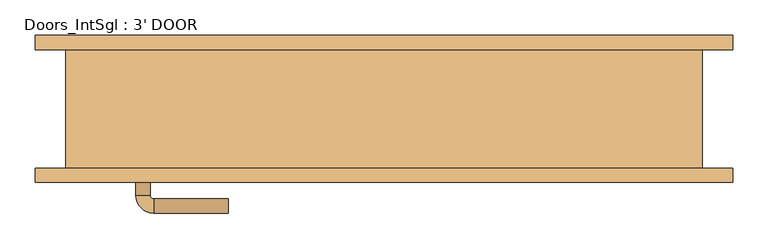
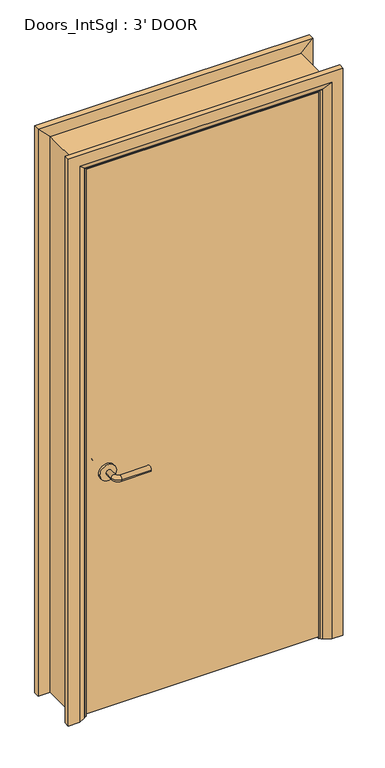
"""IFC4 building model written with IfcOpenShell, lengths in millimetres: door geometry, Doors_IntSgl : 3' DOOR."""

from ifc_helpers import new_model, si_unit, point, frame, frame_2d, origin, place, context, project, spatial, polyline, circle_curve, ellipse_curve, trimmed, segment, composite_curve, outline, extrude, faceted_brep, source, transform, mapped, element, save
from ifc_brep_helpers import plane_surface, cylinder_surface, revolved_surface, advanced_brep


def doors_intsgl_3_door_2f660dd7(model_context):
    return source(origin(), model_context, "Body", "SolidModel", [
        advanced_brep(
        [(-350.2, -37.82, 900.0), (-330.2, -37.82, 900.0), (-350.2, -7.82, 900.0), (-330.2, -7.82, 900.0), (-325.2, -2.82, 900.0), (-325.2, 17.18, 900.0), (-220.2, 17.18, 900.0), (-220.2, -2.82, 900.0)],
        [
            (0, 1, circle_curve(frame((-340.2, -37.82, 900.0), z_axis=(0.0, -1.0, 0.0), x_axis=(1.0, 0.0, 0.0)), 10.0)),
            (1, 0, circle_curve(frame((-340.2, -37.82, 900.0), z_axis=(0.0, -1.0, 0.0), x_axis=(1.0, 0.0, 0.0)), 10.0)),
            (0, 2),
            (2, 3, circle_curve(frame((-340.2, -7.82, 900.0), z_axis=(0.0, -1.0, 0.0), x_axis=(1.0, 0.0, 0.0)), 10.0)),
            (3, 1),
            (3, 2, circle_curve(frame((-340.2, -7.82, 900.0), z_axis=(0.0, -1.0, 0.0), x_axis=(1.0, 0.0, 0.0)), 10.0)),
            (4, 3, circle_curve(frame((-325.2, -7.82, 900.0), z_axis=(0.0, 0.0, 1.0), x_axis=(-1.0, 0.0, 0.0)), 5.0)),
            (2, 5, circle_curve(frame((-325.2, -7.82, 900.0), z_axis=(0.0, 0.0, -1.0), x_axis=(-1.0, 0.0, 0.0)), 25.0)),
            (5, 4, circle_curve(frame((-325.2, 7.18, 900.0), z_axis=(-1.0, 0.0, 0.0), x_axis=(0.0, -1.0, 0.0)), 10.0)),
            (4, 5, circle_curve(frame((-325.2, 7.18, 900.0), z_axis=(-1.0, 0.0, 0.0), x_axis=(0.0, -1.0, 0.0)), 10.0)),
            (6, 7, circle_curve(frame((-220.2, 7.18, 900.0), z_axis=(1.0, 0.0, 0.0), x_axis=(0.0, -1.0, 0.0)), 10.0)),
            (7, 6, circle_curve(frame((-220.2, 7.18, 900.0), z_axis=(1.0, 0.0, 0.0), x_axis=(0.0, -1.0, 0.0)), 10.0)),
            (5, 6),
            (7, 4),
        ],
        [
            plane_surface(frame((-340.2, -37.82, 900.0), z_axis=(0.0, -1.0, 0.0), x_axis=(0.0, 0.0, 1.0))),
            cylinder_surface(frame((-340.2, -37.82, 900.0), z_axis=(0.0, -1.0, 0.0), x_axis=(1.0, 0.0, 0.0)), 10.0),
            revolved_surface(trimmed(ellipse_curve(frame((-340.2, -7.82, 900.0), z_axis=(0.0, -1.0, 0.0), x_axis=(1.0, 0.0, 0.0)), 10.0, 10.0), [point((-350.2, -7.82, 900.0))], [point((-330.2, -7.82, 900.0))], True, "CARTESIAN"), (-325.2, -7.82, 900.0), (0.0, 0.0, -1.0)),
            revolved_surface(trimmed(ellipse_curve(frame((-340.2, -7.82, 900.0), z_axis=(0.0, -1.0, 0.0), x_axis=(1.0, 0.0, 0.0)), 10.0, 10.0), [point((-330.2, -7.82, 900.0))], [point((-350.2, -7.82, 900.0))], True, "CARTESIAN"), (-325.2, -7.82, 900.0), (0.0, 0.0, -1.0)),
            plane_surface(frame((-220.2, 7.18, 900.0), z_axis=(1.0, 0.0, 0.0), x_axis=(0.0, 0.0, 1.0))),
            cylinder_surface(frame((-325.2, 7.18, 900.0), z_axis=(-1.0, 0.0, 0.0), x_axis=(0.0, -1.0, 0.0)), 10.0),
        ],
        [
            (0, [[1, 2]]),
            (1, [[-1, 3, 4, 5]]),
            (1, [[-2, -5, 6, -3]]),
            (2, [[7, -4, 8, 9]]),
            (3, [[-8, -6, -7, 10]]),
            (4, [[11, 12]]),
            (5, [[-9, 13, -12, 14]]),
            (5, [[-10, -14, -11, -13]]),
        ],
    ),
        extrude(outline(composite_curve([segment(trimmed(circle_curve(frame_2d((900.0, -342.7)), 30.0), [point((900.0, -372.7))], [point((900.0, -312.7))], False, "CARTESIAN"), True, "CONTINUOUS"), segment(trimmed(circle_curve(frame_2d((900.0, -342.7)), 30.0), [point((900.0, -312.7))], [point((900.0, -372.7))], False, "CARTESIAN"), True, "CONTINUOUS")], self_intersect=False)), frame((0.0, -45.82, 0.0), z_axis=(0.0, 1.0, 0.0), x_axis=(0.0, 0.0, 1.0)), (0.0, 0.0, 1.0), 8.0),
        advanced_brep(
        [(-350.2, -91.82, 900.0), (-330.2, -91.82, 900.0), (-330.2, -121.82, 900.0), (-350.2, -121.82, 900.0), (-325.2, -126.82, 900.0), (-325.2, -146.82, 900.0), (-220.2, -146.82, 900.0), (-220.2, -126.82, 900.0)],
        [
            (0, 1, circle_curve(frame((-340.2, -91.82, 900.0), z_axis=(0.0, 1.0, 0.0), x_axis=(1.0, 0.0, 0.0)), 10.0)),
            (1, 0, circle_curve(frame((-340.2, -91.82, 900.0), z_axis=(0.0, 1.0, 0.0), x_axis=(1.0, 0.0, 0.0)), 10.0)),
            (1, 2),
            (2, 3, circle_curve(frame((-340.2, -121.82, 900.0), z_axis=(0.0, 1.0, 0.0), x_axis=(1.0, 0.0, 0.0)), 10.0)),
            (3, 0),
            (3, 2, circle_curve(frame((-340.2, -121.82, 900.0), z_axis=(0.0, 1.0, 0.0), x_axis=(1.0, 0.0, 0.0)), 10.0)),
            (4, 5, circle_curve(frame((-325.2, -136.82, 900.0), z_axis=(-1.0, 0.0, 0.0), x_axis=(0.0, 1.0, 0.0)), 10.0)),
            (5, 3, circle_curve(frame((-325.2, -121.82, 900.0), z_axis=(0.0, 0.0, -1.0), x_axis=(-1.0, 0.0, 0.0)), 25.0)),
            (2, 4, circle_curve(frame((-325.2, -121.82, 900.0), z_axis=(0.0, 0.0, 1.0), x_axis=(-1.0, 0.0, 0.0)), 5.0)),
            (5, 4, circle_curve(frame((-325.2, -136.82, 900.0), z_axis=(-1.0, 0.0, 0.0), x_axis=(0.0, 1.0, 0.0)), 10.0)),
            (6, 7, circle_curve(frame((-220.2, -136.82, 900.0), z_axis=(1.0, 0.0, 0.0), x_axis=(0.0, 1.0, 0.0)), 10.0)),
            (7, 6, circle_curve(frame((-220.2, -136.82, 900.0), z_axis=(1.0, 0.0, 0.0), x_axis=(0.0, 1.0, 0.0)), 10.0)),
            (4, 7),
            (6, 5),
        ],
        [
            plane_surface(frame((-340.2, -91.82, 900.0), z_axis=(0.0, 1.0, 0.0), x_axis=(0.0, 0.0, 1.0))),
            cylinder_surface(frame((-340.2, -91.82, 900.0), z_axis=(0.0, 1.0, 0.0), x_axis=(1.0, 0.0, 0.0)), 10.0),
            revolved_surface(trimmed(ellipse_curve(frame((-340.2, -121.82, 900.0), z_axis=(0.0, -1.0, 0.0), x_axis=(1.0, 0.0, 0.0)), 10.0, 10.0), [point((-350.2, -121.82, 900.0))], [point((-330.2, -121.82, 900.0))], True, "CARTESIAN"), (-325.2, -121.82, 900.0), (0.0, 0.0, -1.0)),
            revolved_surface(trimmed(ellipse_curve(frame((-340.2, -121.82, 900.0), z_axis=(0.0, -1.0, 0.0), x_axis=(1.0, 0.0, 0.0)), 10.0, 10.0), [point((-330.2, -121.82, 900.0))], [point((-350.2, -121.82, 900.0))], True, "CARTESIAN"), (-325.2, -121.82, 900.0), (0.0, 0.0, -1.0)),
            plane_surface(frame((-220.2, -136.82, 900.0), z_axis=(1.0, 0.0, 0.0), x_axis=(0.0, 0.0, 1.0))),
            cylinder_surface(frame((-325.2, -136.82, 900.0), z_axis=(-1.0, 0.0, 0.0), x_axis=(0.0, 1.0, 0.0)), 10.0),
        ],
        [
            (0, [[1, 2]]),
            (1, [[3, 4, 5, -2]]),
            (1, [[-5, 6, -3, -1]]),
            (2, [[7, 8, -4, 9]]),
            (3, [[10, -9, -6, -8]]),
            (4, [[11, 12]]),
            (5, [[13, -11, 14, -7]]),
            (5, [[-14, -12, -13, -10]]),
        ],
    ),
        extrude(outline(composite_curve([segment(trimmed(circle_curve(frame_2d((900.0, -342.7)), 30.0), [point((900.0, -372.7))], [point((900.0, -312.7))], False, "CARTESIAN"), True, "CONTINUOUS"), segment(trimmed(circle_curve(frame_2d((900.0, -342.7)), 30.0), [point((900.0, -312.7))], [point((900.0, -372.7))], False, "CARTESIAN"), True, "CONTINUOUS")], self_intersect=False)), frame((0.0, -91.82, 0.0), z_axis=(0.0, 1.0, 0.0), x_axis=(0.0, 0.0, 1.0)), (0.0, 0.0, 1.0), 8.0),
        extrude(outline(polyline([(415.2, -45.82), (415.2, -83.82), (-415.2, -83.82), (-415.2, -45.82), (415.2, -45.82)])), frame((0.0, 0.0, 8.0), z_axis=(0.0, 0.0, 1.0), x_axis=(1.0, 0.0, 0.0)), (0.0, 0.0, 1.0), 2060.0),
        advanced_brep(
        [(492.2, -103.82, 0.0), (452.2, -103.82, 0.0), (426.2, -89.82, 0.0), (422.2, -83.82, 0.0), (492.2, -83.82, 0.0), (492.2, -83.82, 2145.0), (492.2, -103.82, 2145.0), (422.2, -83.82, 2075.0), (-422.2, -83.82, 2075.0), (-422.2, -83.82, 0.0), (-492.2, -83.82, 0.0), (-492.2, -83.82, 2145.0), (426.2, -89.82, 2079.0), (452.2, -103.82, 2105.0), (-492.2, -103.82, 2145.0), (-492.2, -103.82, 0.0), (-452.2, -103.82, 0.0), (-452.2, -103.82, 2105.0), (-426.2, -89.82, 0.0), (-426.2, -89.82, 2079.0)],
        [
            (0, 1),
            (1, 2),
            (2, 3, circle_curve(frame((430.2, -82.82, 0.0), z_axis=(0.0, 0.0, -1.0), x_axis=(1.0, 0.0, 0.0)), 8.0622577)),
            (3, 4),
            (4, 0),
            (4, 5),
            (5, 6),
            (6, 0),
            (3, 7),
            (7, 8),
            (8, 9),
            (9, 10),
            (10, 11),
            (11, 5),
            (2, 12),
            (12, 7, ellipse_curve(frame((430.2, -82.82, 2083.0), z_axis=(0.7071067811865475, 0.0, -0.7071067811865475), x_axis=(-0.7071067811865474, 0.0, -0.7071067811865476)), 11.4017543, 8.0622577)),
            (1, 13),
            (13, 12),
            (6, 14),
            (14, 15),
            (15, 16),
            (16, 17),
            (17, 13),
            (10, 15),
            (14, 11),
            (9, 18, circle_curve(frame((-430.2, -82.82, 0.0), z_axis=(0.0, 0.0, -1.0), x_axis=(-1.0, 0.0, 0.0)), 8.0622577)),
            (18, 16),
            (19, 18),
            (8, 19, ellipse_curve(frame((-430.2, -82.82, 2083.0), z_axis=(-0.7071067811865475, 0.0, -0.7071067811865475), x_axis=(-0.7071067811865474, 0.0, 0.7071067811865476)), 11.4017543, 8.0622577)),
            (19, 17),
            (12, 19),
        ],
        [
            plane_surface(frame((422.2, -83.82, 0.0), z_axis=(0.0, 0.0, -1.0), x_axis=(0.0, 1.0, 0.0))),
            plane_surface(frame((492.2, -103.82, 0.0), z_axis=(1.0, 0.0, 0.0), x_axis=(0.0, 0.0, 1.0))),
            plane_surface(frame((492.2, -83.82, 0.0), z_axis=(0.0, 1.0, 0.0), x_axis=(0.0, 0.0, 1.0))),
            cylinder_surface(frame((430.2, -82.82, 0.0), z_axis=(0.0, 0.0, -1.0), x_axis=(1.0, 0.0, 0.0)), 8.0622577),
            plane_surface(frame((426.2, -89.82, 0.0), z_axis=(-0.4740998230350126, -0.880471099922178, 0.0), x_axis=(0.0, 0.0, 1.0))),
            plane_surface(frame((452.2, -103.82, 0.0), z_axis=(0.0, -1.0, 0.0), x_axis=(0.0, 0.0, 1.0))),
            plane_surface(frame((-492.2, -103.82, 2145.0), z_axis=(-1.0, 0.0, 0.0), x_axis=(0.0, 0.0, -1.0))),
            plane_surface(frame((-422.2, -83.82, 0.0), z_axis=(0.0, 0.0, -1.0), x_axis=(0.0, 1.0, 0.0))),
            cylinder_surface(frame((-430.2, -82.82, 2075.0), z_axis=(0.0, 0.0, 1.0), x_axis=(-1.0, 0.0, 0.0)), 8.0622577),
            plane_surface(frame((-426.2, -89.82, 2079.0), z_axis=(0.47409982303501824, -0.8804710999221749, 0.0), x_axis=(0.0, 0.0, -1.0))),
            plane_surface(frame((492.2, -103.82, 2145.0), z_axis=(0.0, 0.0, 1.0), x_axis=(-1.0, 0.0, 0.0))),
            cylinder_surface(frame((422.2, -82.82, 2083.0), z_axis=(1.0, 0.0, 0.0), x_axis=(0.0, 0.0, 1.0)), 8.0622577),
            plane_surface(frame((426.2, -89.82, 2079.0), z_axis=(0.0, -0.8804710999221764, -0.4740998230350154), x_axis=(-1.0, 0.0, 0.0))),
        ],
        [
            (0, [[1, 2, 3, 4, 5]]),
            (1, [[6, 7, 8, -5]]),
            (2, [[9, 10, 11, 12, 13, 14, -6, -4]]),
            (3, [[15, 16, -9, -3]]),
            (4, [[17, 18, -15, -2]]),
            (5, [[-8, 19, 20, 21, 22, 23, -17, -1]]),
            (6, [[-13, 24, -20, 25]]),
            (7, [[-24, -12, 26, 27, -21]]),
            (8, [[28, -26, -11, 29]]),
            (9, [[-22, -27, -28, 30]]),
            (10, [[-14, -25, -19, -7]]),
            (11, [[31, -29, -10, -16]]),
            (12, [[-23, -30, -31, -18]]),
        ],
    ),
        extrude(outline(polyline([(0.0, -398.2), (2051.0, -398.2), (2051.0, 398.2), (0.0, 398.2), (0.0, 417.2), (2070.0, 417.2), (2070.0, -417.2), (0.0, -417.2), (0.0, -398.2)])), frame((0.0, -43.82, 0.0), z_axis=(0.0, 1.0, 0.0), x_axis=(0.0, 0.0, 1.0)), (0.0, 0.0, 1.0), 32.0),
        advanced_brep(
        [(-492.2, 103.82, 0.0), (-452.2, 103.82, 0.0), (-426.2, 89.82, 0.0), (-422.2, 83.82, 0.0), (-492.2, 83.82, 0.0), (-492.2, 83.82, 2145.0), (-492.2, 103.82, 2145.0), (-422.2, 83.82, 2075.0), (-426.2, 89.82, 2079.0), (-452.2, 103.82, 2105.0), (492.2, 103.82, 0.0), (492.2, 83.82, 0.0), (422.2, 83.82, 0.0), (426.2, 89.82, 0.0), (452.2, 103.82, 0.0), (492.2, 103.82, 2145.0), (452.2, 103.82, 2105.0), (426.2, 89.82, 2079.0), (422.2, 83.82, 2075.0), (492.2, 83.82, 2145.0)],
        [
            (0, 1),
            (1, 2),
            (2, 3, circle_curve(frame((-430.2, 82.82, 0.0), z_axis=(0.0, 0.0, -1.0), x_axis=(-1.0, 0.0, 0.0)), 8.0622577)),
            (3, 4),
            (4, 0),
            (4, 5),
            (5, 6),
            (6, 0),
            (3, 7),
            (7, 5),
            (2, 8),
            (8, 7, ellipse_curve(frame((-430.2, 82.82, 2083.0), z_axis=(-0.7071067811865475, 0.0, -0.7071067811865475), x_axis=(0.7071067811865474, 0.0, -0.7071067811865476)), 11.4017543, 8.0622577)),
            (1, 9),
            (9, 8),
            (6, 9),
            (10, 11),
            (11, 12),
            (12, 13, circle_curve(frame((430.2, 82.82, 0.0), z_axis=(0.0, 0.0, -1.0), x_axis=(1.0, 0.0, 0.0)), 8.0622577)),
            (13, 14),
            (14, 10),
            (15, 10),
            (14, 16),
            (16, 15),
            (13, 17),
            (17, 16),
            (12, 18),
            (18, 17, ellipse_curve(frame((430.2, 82.82, 2083.0), z_axis=(0.7071067811865475, 0.0, -0.7071067811865475), x_axis=(0.7071067811865474, 0.0, 0.7071067811865476)), 11.4017543, 8.0622577)),
            (11, 19),
            (19, 18),
            (15, 19),
            (5, 19),
            (15, 6),
            (7, 18),
            (8, 17),
            (9, 16),
        ],
        [
            plane_surface(frame((-422.2, 156.6210989, 0.0), z_axis=(0.0, 0.0, -1.0), x_axis=(1.0, 0.0, 0.0))),
            plane_surface(frame((-492.2, 103.82, 0.0), z_axis=(-1.0, 0.0, 0.0), x_axis=(0.0, 0.0, 1.0))),
            plane_surface(frame((-492.2, 83.82, 0.0), z_axis=(0.0, -1.0, 0.0), x_axis=(0.0, 0.0, 1.0))),
            cylinder_surface(frame((-430.2, 82.82, 0.0), z_axis=(0.0, 0.0, -1.0), x_axis=(-1.0, 0.0, 0.0)), 8.0622577),
            plane_surface(frame((-426.2, 89.82, 0.0), z_axis=(0.4740998230350183, 0.8804710999221749, 0.0), x_axis=(0.0, 0.0, 1.0))),
            plane_surface(frame((-452.2, 103.82, 0.0), z_axis=(0.0, 1.0, 0.0), x_axis=(0.0, 0.0, 1.0))),
            plane_surface(frame((422.2, 156.6210989, 0.0), z_axis=(0.0, 0.0, -1.0), x_axis=(-1.0, 0.0, 0.0))),
            plane_surface(frame((452.2, 103.82, 2105.0), z_axis=(0.0, 1.0, 0.0), x_axis=(0.0, 0.0, -1.0))),
            plane_surface(frame((426.2, 89.82, 2079.0), z_axis=(-0.4740998230350183, 0.8804710999221749, 0.0), x_axis=(0.0, 0.0, -1.0))),
            cylinder_surface(frame((430.2, 82.82, 2075.0), z_axis=(0.0, 0.0, 1.0), x_axis=(1.0, 0.0, 0.0)), 8.0622577),
            plane_surface(frame((492.2, 83.82, 2145.0), z_axis=(0.0, -1.0, 0.0), x_axis=(0.0, 0.0, -1.0))),
            plane_surface(frame((492.2, 103.82, 2145.0), z_axis=(1.0, 0.0, 0.0), x_axis=(0.0, 0.0, -1.0))),
            plane_surface(frame((-492.2, 103.82, 2145.0), z_axis=(0.0, 0.0, 1.0), x_axis=(1.0, 0.0, 0.0))),
            plane_surface(frame((-492.2, 83.82, 2145.0), z_axis=(0.0, -1.0, 0.0), x_axis=(1.0, 0.0, 0.0))),
            cylinder_surface(frame((-422.2, 82.82, 2083.0), z_axis=(-1.0, 0.0, 0.0), x_axis=(0.0, 0.0, 1.0)), 8.0622577),
            plane_surface(frame((-426.2, 89.82, 2079.0), z_axis=(0.0, 0.8804710999221749, -0.4740998230350183), x_axis=(1.0, 0.0, 0.0))),
            plane_surface(frame((-452.2, 103.82, 2105.0), z_axis=(0.0, 1.0, 0.0), x_axis=(1.0, 0.0, 0.0))),
        ],
        [
            (0, [[1, 2, 3, 4, 5]]),
            (1, [[6, 7, 8, -5]]),
            (2, [[9, 10, -6, -4]]),
            (3, [[11, 12, -9, -3]]),
            (4, [[13, 14, -11, -2]]),
            (5, [[-8, 15, -13, -1]]),
            (6, [[16, 17, 18, 19, 20]]),
            (7, [[21, -20, 22, 23]]),
            (8, [[-22, -19, 24, 25]]),
            (9, [[-24, -18, 26, 27]]),
            (10, [[-26, -17, 28, 29]]),
            (11, [[-28, -16, -21, 30]]),
            (12, [[31, -30, 32, -7]]),
            (13, [[33, -29, -31, -10]]),
            (14, [[34, -27, -33, -12]]),
            (15, [[35, -25, -34, -14]]),
            (16, [[-32, -23, -35, -15]]),
        ],
    ),
        faceted_brep([(-417.2, -83.82, 0.0), (-449.2, -83.82, 0.0), (-449.2, 83.82, 0.0), (-417.2, 83.82, 0.0), (-417.2, 83.82, 2070.0), (-417.2, -83.82, 2070.0), (-449.2, 83.82, 2102.0), (-449.2, -83.82, 2102.0), (417.2, -83.82, 0.0), (417.2, 83.82, 0.0), (449.2, 83.82, 0.0), (449.2, -83.82, 0.0), (417.2, -83.82, 2070.0), (449.2, -83.82, 2102.0), (449.2, 83.82, 2102.0), (417.2, 83.82, 2070.0)], [[[0, 1, 2, 3]], [[3, 4, 5, 0]], [[2, 6, 4, 3]], [[1, 7, 6, 2]], [[0, 5, 7, 1]], [[8, 9, 10, 11]], [[12, 8, 11, 13]], [[13, 11, 10, 14]], [[14, 10, 9, 15]], [[15, 9, 8, 12]], [[4, 15, 12, 5]], [[6, 14, 15, 4]], [[7, 13, 14, 6]], [[5, 12, 13, 7]]]),
    ])


if __name__ == "__main__":
    model = new_model("IFC4")
    model_context = context("Model", 3, world=origin())
    ifc_project = project(units=[si_unit("LENGTHUNIT", "METRE", prefix="MILLI")], contexts=[model_context])
    site = spatial("IfcSite", under=ifc_project)
    building = spatial("IfcBuilding", under=site)
    placement = place(None, origin())
    doors_intsgl_3_door_shape = doors_intsgl_3_door_2f660dd7(model_context)
    element("IfcDoor", 1, ObjectType="Doors_IntSgl : 3' DOOR", at=placement, inside=building, context=model_context, shape_type="MappedRepresentation", body=[
        mapped(doors_intsgl_3_door_shape, transform((0.0, 0.0, 0.0), x_axis=(1.0, 0.0, 0.0), y_axis=(0.0, 1.0, 0.0), z_axis=(0.0, 0.0, 1.0))),
    ])
    save(model, "model.ifc")

# Revit data of these elements
# Type "Doors_IntSgl : 3' DOOR"
#   Type Mark = "46"
#   Type Comments = "Internal Single"
#   Operation = "SingleSwingRight"
#   Manufacturer = "Revit"
#   Keynote = "L20"
#   Description = "Internal Single Door"
#   Analytic Construction = "Metal"
#   UnderCut = 0.026247 ft
#   Tolerance = 0.006562 ft
#   Thickness = 0.124672 ft
#   Thermal Resistance (R) = 0.270117 (m²·K)/W
#   Structural Tolerance = 0.026247 ft
#   StopDepth = 0.104987 ft
#   Stop Thickness = 0.062336 ft
#   Rough Width = 3.0 ft
#   Rough Height = 6.922572 ft
#   Height to Top Lock Rail = 3.28084 ft
#   Heat Transfer Coefficient (U) = 3.7021 W/(m²·K)
#   Handle Z Distance = 2.952756 ft
#   Handle X Distance = 0.246063 ft
#   Frame Thickness = 0.104987 ft
#   Door Panel Width = 2.724409 ft
#   Door Panel Thickness = 0.124672 ft
#   Door Panel Offset = 0.0 ft
#   Height = 6.922572 ft
#   Width = 3.0 ft
#   Door Panel Height = 6.75853 ft
#   Architrave Setback = 0.016404 ft
#   Vis - Ironmongery = yes
#   Material Ironmongery = Door - Handle
#   Material Frame = Door - Frame/Mullion (1)
#   Material Door = Door - Panel
#   Material Architrave = Door - Architrave
#   Visual Light Transmittance = 0
#   Solar Heat Gain Coefficient = 0
#   Function = (empty or 0)
#   Wall Closure = (empty or 0)
# Element 1 (IfcDoor, "Doors_IntSgl : 3' DOOR")
#   Materials on its faces: "Door - Architrave", "Door - Handle", "Door - Frame/Mullion (1)", "Door - Panel"
# Materials
#   "Door - Handle": colour RGB 0 0 0, transparency 0, Keynote = "P21", Cost = 0
#   "Door - Frame/Mullion (1)": class "Wood", colour RGB 212 179 113, transparency 0, Keynote = "L20", Cost = 0
#   "Door - Panel": class "Wood", colour RGB 210 159 95, transparency 0, Keynote = "L20", Cost = 0
#   "Door - Architrave": class "Wood", colour RGB 154 90 5, transparency 0, Keynote = "P20", Cost = 0
